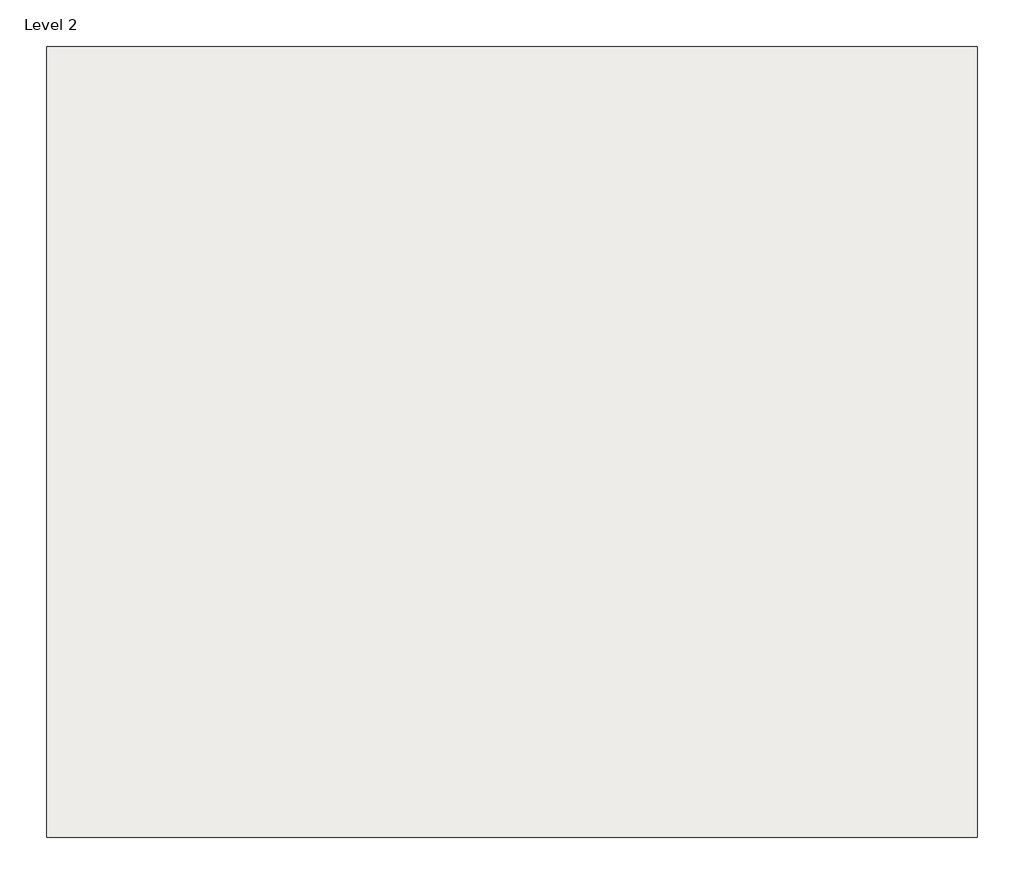
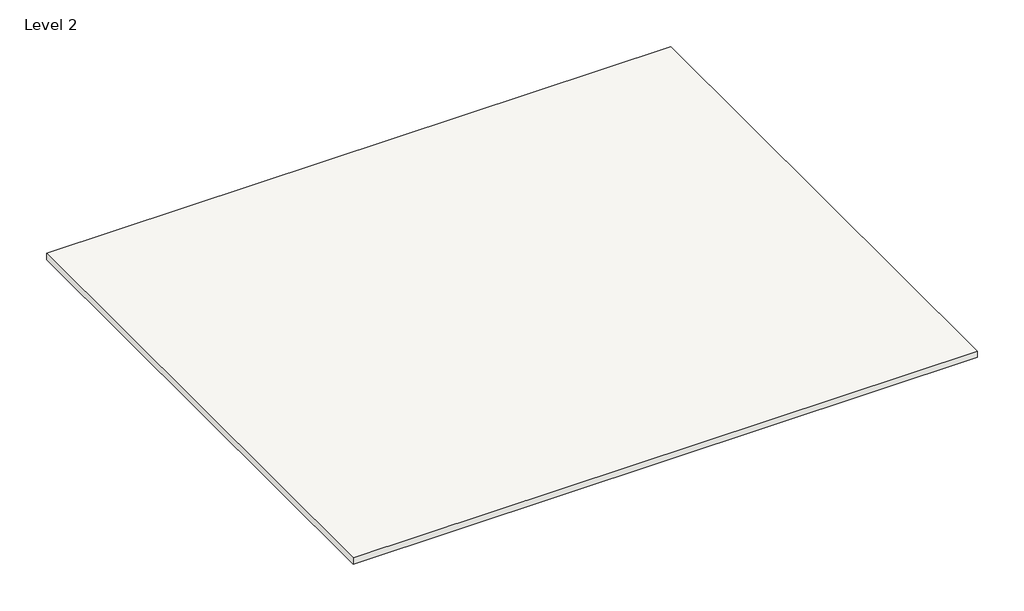
# One storey: 1 slab.
"""IFC4 building model written with IfcOpenShell, lengths in millimetres."""

from ifc_helpers import new_model, si_unit, frame, origin, place, context, project, spatial, polyline, outline, extrude, element, save

model = new_model("IFC4")

# Units and contexts
model_context = context("Model", 3, world=origin())
ifc_project = project(units=[si_unit("LENGTHUNIT", "METRE", prefix="MILLI")], contexts=[model_context])

# Site, building, storey
site = spatial("IfcSite", under=ifc_project)
building = spatial("IfcBuilding", under=site)
storey = spatial("IfcBuildingStorey", under=building, Name="Level 2", Elevation=3657.6)

# Slab
placement = place(None, origin())
element("IfcSlab", 1, ObjectType="6\" GF", at=placement, inside=storey, context=model_context, shape_type="SweptSolid", body=[
    extrude(outline(polyline([(5532.2756121, 8667.6116878), (5532.2756121, -3143.3883122), (-8361.5243879, -3143.3883122), (-8361.5243879, 8667.6116878), (5532.2756121, 8667.6116878)])), frame((0.0, 0.0, 3657.6), z_axis=(0.0, 0.0, 1.0), x_axis=(1.0, 0.0, 0.0)), (0.0, 0.0, 1.0), 152.4),
])

save(model, "model.ifc")

# Revit data of these elements
# Type "6\" GF"
#   Assembly Code = "B1010"
#   Function = 0
#   Layers, outside or top first: 0' - 6" no material (function 1)
# Element 1 (IfcSlab, "6\" GF")
#   Height Offset From Level = 0' - 6"
#   Phase Created = New Construction
#   Materials on its faces: "Default Floor"
# Materials
#   "Default Floor": colour RGB 128 128 128, transparency 0, Cost = 0
